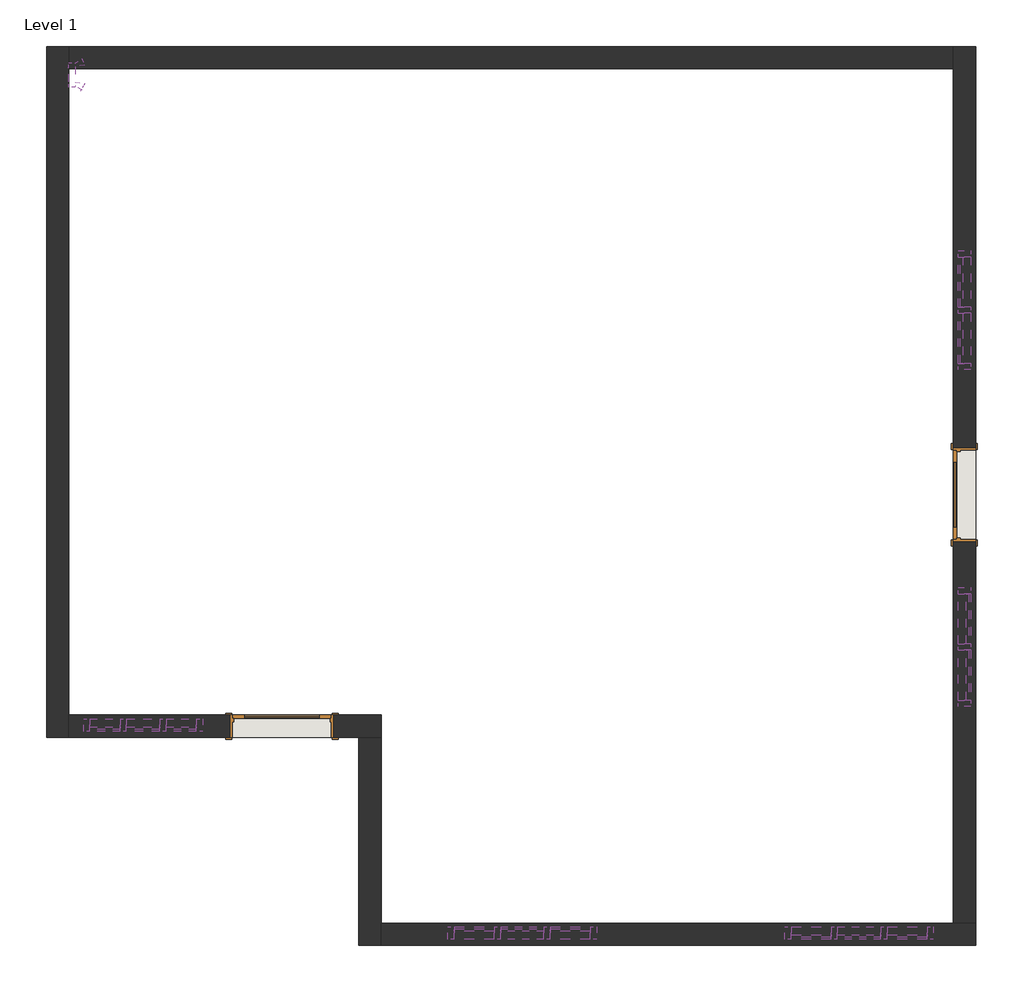
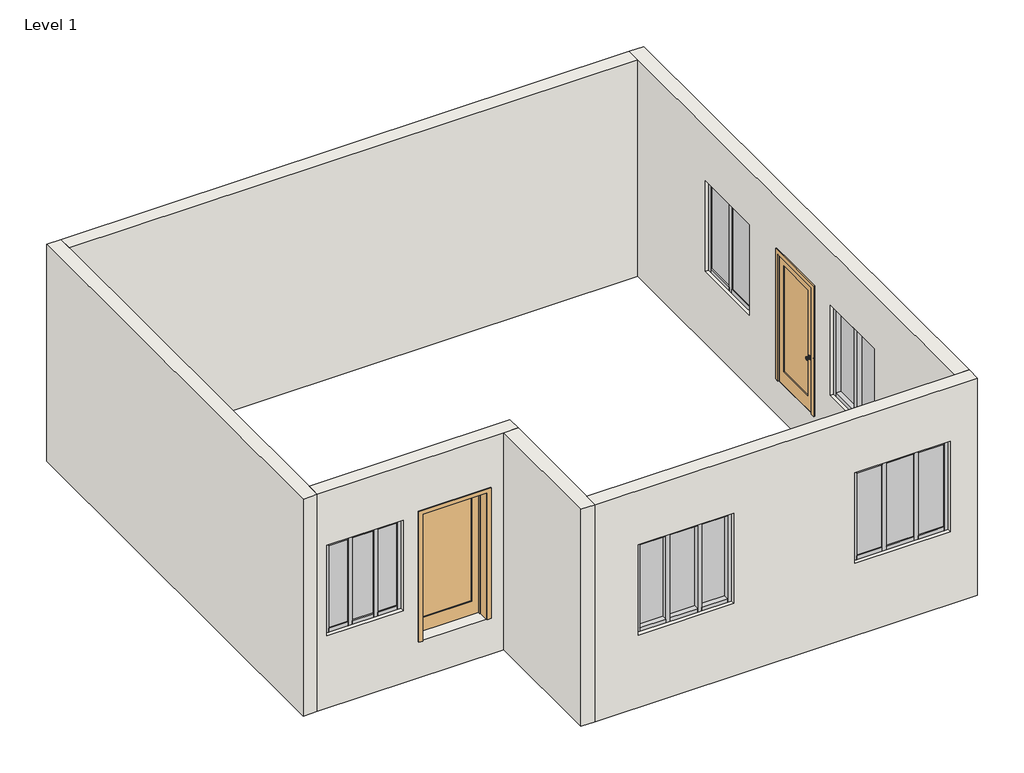
# One storey: 44 members, 13 plates, 6 walls, 2 doors, 1 light fixture.
"""IFC4 building model written with IfcOpenShell, lengths in millimetres."""

from ifc_helpers import new_model, si_unit, frame, origin, place, context, project, spatial, polyline, outline, extrude, faceted_brep, transform, mapped, element, save
from components import door_3b97b8e7, door_3a9a63a9, emergency_wall_light_120v_c8ddf26d, member_5ad95953, member_82905deb, member_ff1b7d8f, member_4491d118, member_dc106669, member_bc7dbe04, member_0b7646a3, system_panel_glazed_3ea5ab3e, system_panel_glazed_321d670a, system_panel_glazed_d22dc6a9, system_panel_glazed_17c4a998, system_panel_glazed_24803b90

model = new_model("IFC4")

# Units and contexts
model_context = context("Model", 3, world=origin())
ifc_project = project(units=[si_unit("LENGTHUNIT", "METRE", prefix="MILLI")], contexts=[model_context])

# Site, building, storey
site = spatial("IfcSite", under=ifc_project)
building = spatial("IfcBuilding", under=site)
storey = spatial("IfcBuildingStorey", under=building, Name="Level 1", Elevation=-609.6)

# Doors
placement = place(None, origin())
door_shape = door_3b97b8e7(model_context)
element("IfcDoor", 1, ObjectType="Door-Interior-Single-1_Panel-Wood : 36\" x 84\" 3", at=placement, inside=storey, context=model_context, shape_type="MappedRepresentation", body=[
    mapped(door_shape, transform((-1873.6852438, 78.3065419, 0.0), x_axis=(0.0, 1.0, 0.0), y_axis=(-1.0, 0.0, 0.0), z_axis=(0.0, 0.0, 1.0))),
])
door_2_shape = door_3a9a63a9(model_context)
element("IfcDoor", 2, ObjectType="Door-Interior-Single-1_Panel-Wood : 40\" x 84\"", at=placement, inside=storey, context=model_context, shape_type="MappedRepresentation", body=[
    mapped(door_2_shape, transform((-8868.2102438, -2293.4184581, 0.0), x_axis=(1.0, 0.0, 0.0), y_axis=(0.0, 1.0, 0.0), z_axis=(0.0, 0.0, 1.0))),
])

# Light fixture
emergency_wall_light_120v_shape = emergency_wall_light_120v_c8ddf26d(model_context)
element("IfcLightFixture", 3, ObjectType="Emergency Wall Light : 120V", at=placement, inside=storey, context=model_context, shape_type="MappedRepresentation", body=[
    mapped(emergency_wall_light_120v_shape, transform((-11195.7738092, 4383.6065419, 301.1463629), x_axis=(0.0, -1.0, 0.0), y_axis=(1.0, 0.0, 0.0), z_axis=(0.0, 0.0, 1.0))),
])

# Members
member_shape = member_5ad95953(model_context)
element("IfcMember", 4, ObjectType="Rectangular Mullion : 2.5\" x 5\" rectangular", at=placement, inside=storey, context=model_context, shape_type="MappedRepresentation", body=[
    mapped(member_shape, transform((-10836.7102438, -2283.8934581, 2133.6), x_axis=(0.0, 0.0, 1.0), y_axis=(0.0, 1.0, 0.0), z_axis=(-1.0, 0.0, 0.0))),
])
element("IfcMember", 5, ObjectType="Rectangular Mullion : 2.5\" x 5\" rectangular", at=placement, inside=storey, context=model_context, shape_type="MappedRepresentation", body=[
    mapped(member_shape, transform((-10055.6602438, -2283.8934581, 2133.6), x_axis=(0.0, 0.0, 1.0), y_axis=(0.0, 1.0, 0.0), z_axis=(-1.0, 0.0, 0.0))),
])
element("IfcMember", 6, ObjectType="Rectangular Mullion : 2.5\" x 5\" rectangular", at=placement, inside=storey, context=model_context, shape_type="MappedRepresentation", body=[
    mapped(member_shape, transform((-9744.5102438, -2283.8934581, 609.6), x_axis=(0.0, 0.0, -1.0), y_axis=(0.0, 1.0, 0.0), z_axis=(1.0, 0.0, 0.0))),
])
element("IfcMember", 7, ObjectType="Rectangular Mullion : 2.5\" x 5\" rectangular", at=placement, inside=storey, context=model_context, shape_type="MappedRepresentation", body=[
    mapped(member_shape, transform((-10525.5602438, -2283.8934581, 609.6), x_axis=(0.0, 0.0, -1.0), y_axis=(0.0, 1.0, 0.0), z_axis=(1.0, 0.0, 0.0))),
])
member_2_shape = member_82905deb(model_context)
element("IfcMember", 8, ObjectType="Rectangular Mullion : 2.5\" x 5\" rectangular", at=placement, inside=storey, context=model_context, shape_type="MappedRepresentation", body=[
    mapped(member_2_shape, transform((-10493.8102438, -2283.8934581, 609.6), x_axis=(-1.0, 0.0, 0.0), y_axis=(0.0, 1.0, 0.0), z_axis=(0.0, 0.0, -1.0))),
])
element("IfcMember", 9, ObjectType="Rectangular Mullion : 2.5\" x 5\" rectangular", at=placement, inside=storey, context=model_context, shape_type="MappedRepresentation", body=[
    mapped(member_2_shape, transform((-10087.4102438, -2283.8934581, 609.6), x_axis=(-1.0, 0.0, 0.0), y_axis=(0.0, 1.0, 0.0), z_axis=(0.0, 0.0, -1.0))),
])
element("IfcMember", 10, ObjectType="Rectangular Mullion : 2.5\" x 5\" rectangular", at=placement, inside=storey, context=model_context, shape_type="MappedRepresentation", body=[
    mapped(member_2_shape, transform((-6658.4102438, -4417.4934581, 609.6), x_axis=(1.0, 0.0, 0.0), y_axis=(0.0, -1.0, 0.0), z_axis=(0.0, 0.0, -1.0))),
])
element("IfcMember", 11, ObjectType="Rectangular Mullion : 2.5\" x 5\" rectangular", at=placement, inside=storey, context=model_context, shape_type="MappedRepresentation", body=[
    mapped(member_2_shape, transform((-6150.4102438, -4417.4934581, 609.6), x_axis=(1.0, 0.0, 0.0), y_axis=(0.0, -1.0, 0.0), z_axis=(0.0, 0.0, -1.0))),
])
element("IfcMember", 12, ObjectType="Rectangular Mullion : 2.5\" x 5\" rectangular", at=placement, inside=storey, context=model_context, shape_type="MappedRepresentation", body=[
    mapped(member_2_shape, transform((-3204.0102438, -4417.4934581, 609.6), x_axis=(-1.0, 0.0, 0.0), y_axis=(0.0, 1.0, 0.0), z_axis=(0.0, 0.0, -1.0))),
])
element("IfcMember", 13, ObjectType="Rectangular Mullion : 2.5\" x 5\" rectangular", at=placement, inside=storey, context=model_context, shape_type="MappedRepresentation", body=[
    mapped(member_2_shape, transform((-2696.0102438, -4417.4934581, 609.6), x_axis=(-1.0, 0.0, 0.0), y_axis=(0.0, 1.0, 0.0), z_axis=(0.0, 0.0, -1.0))),
])
element("IfcMember", 14, ObjectType="Rectangular Mullion : 2.5\" x 5\" rectangular", at=placement, inside=storey, context=model_context, shape_type="MappedRepresentation", body=[
    mapped(member_2_shape, transform((-1870.5102438, -1483.7934581, 609.6), x_axis=(0.0, -1.0, 0.0), y_axis=(-1.0, 0.0, 0.0), z_axis=(0.0, 0.0, -1.0))),
])
element("IfcMember", 15, ObjectType="Rectangular Mullion : 2.5\" x 5\" rectangular", at=placement, inside=storey, context=model_context, shape_type="MappedRepresentation", body=[
    mapped(member_2_shape, transform((-1870.5102438, 1970.6065419, 609.6), x_axis=(0.0, 1.0, 0.0), y_axis=(1.0, 0.0, 0.0), z_axis=(0.0, 0.0, -1.0))),
])
member_3_shape = member_ff1b7d8f(model_context)
element("IfcMember", 16, ObjectType="Rectangular Mullion : 2.5\" x 5\" rectangular", at=placement, inside=storey, context=model_context, shape_type="MappedRepresentation", body=[
    mapped(member_3_shape, transform((-10119.1602438, -2283.8934581, 609.6), x_axis=(0.0, 0.0, -1.0), y_axis=(0.0, 1.0, 0.0), z_axis=(1.0, 0.0, 0.0))),
])
element("IfcMember", 17, ObjectType="Rectangular Mullion : 2.5\" x 5\" rectangular", at=placement, inside=storey, context=model_context, shape_type="MappedRepresentation", body=[
    mapped(member_3_shape, transform((-10462.0602438, -2283.8934581, 2133.6), x_axis=(0.0, 0.0, 1.0), y_axis=(0.0, 1.0, 0.0), z_axis=(-1.0, 0.0, 0.0))),
])
member_4_shape = member_4491d118(model_context)
element("IfcMember", 18, ObjectType="Rectangular Mullion : 2.5\" x 5\" rectangular", at=placement, inside=storey, context=model_context, shape_type="MappedRepresentation", body=[
    mapped(member_4_shape, transform((-9681.0102438, -2283.8934581, 2133.6), x_axis=(1.0, 0.0, 0.0), y_axis=(0.0, 1.0, 0.0), z_axis=(0.0, 0.0, 1.0))),
])
element("IfcMember", 19, ObjectType="Rectangular Mullion : 2.5\" x 5\" rectangular", at=placement, inside=storey, context=model_context, shape_type="MappedRepresentation", body=[
    mapped(member_4_shape, transform((-7166.4102438, -4417.4934581, 2133.6), x_axis=(-1.0, 0.0, 0.0), y_axis=(0.0, -1.0, 0.0), z_axis=(0.0, 0.0, 1.0))),
])
element("IfcMember", 20, ObjectType="Rectangular Mullion : 2.5\" x 5\" rectangular", at=placement, inside=storey, context=model_context, shape_type="MappedRepresentation", body=[
    mapped(member_4_shape, transform((-2188.0102438, -4417.4934581, 2133.6), x_axis=(1.0, 0.0, 0.0), y_axis=(0.0, 1.0, 0.0), z_axis=(0.0, 0.0, 1.0))),
])
element("IfcMember", 21, ObjectType="Rectangular Mullion : 2.5\" x 5\" rectangular", at=placement, inside=storey, context=model_context, shape_type="MappedRepresentation", body=[
    mapped(member_4_shape, transform((-1870.5102438, -874.1934581, 2133.6), x_axis=(0.0, 1.0, 0.0), y_axis=(-1.0, 0.0, 0.0), z_axis=(0.0, 0.0, 1.0))),
])
element("IfcMember", 22, ObjectType="Rectangular Mullion : 2.5\" x 5\" rectangular", at=placement, inside=storey, context=model_context, shape_type="MappedRepresentation", body=[
    mapped(member_4_shape, transform((-1870.5102438, 1361.0065419, 2133.6), x_axis=(0.0, -1.0, 0.0), y_axis=(1.0, 0.0, 0.0), z_axis=(0.0, 0.0, 1.0))),
])
element("IfcMember", 23, ObjectType="Rectangular Mullion : 2.5\" x 5\" rectangular", at=placement, inside=storey, context=model_context, shape_type="MappedRepresentation", body=[
    mapped(member_4_shape, transform((-10900.2102438, -2283.8934581, 609.6), x_axis=(-1.0, 0.0, 0.0), y_axis=(0.0, 1.0, 0.0), z_axis=(0.0, 0.0, -1.0))),
])
element("IfcMember", 24, ObjectType="Rectangular Mullion : 2.5\" x 5\" rectangular", at=placement, inside=storey, context=model_context, shape_type="MappedRepresentation", body=[
    mapped(member_4_shape, transform((-5642.4102438, -4417.4934581, 609.6), x_axis=(1.0, 0.0, 0.0), y_axis=(0.0, -1.0, 0.0), z_axis=(0.0, 0.0, -1.0))),
])
element("IfcMember", 25, ObjectType="Rectangular Mullion : 2.5\" x 5\" rectangular", at=placement, inside=storey, context=model_context, shape_type="MappedRepresentation", body=[
    mapped(member_4_shape, transform((-3712.0102438, -4417.4934581, 609.6), x_axis=(-1.0, 0.0, 0.0), y_axis=(0.0, 1.0, 0.0), z_axis=(0.0, 0.0, -1.0))),
])
element("IfcMember", 26, ObjectType="Rectangular Mullion : 2.5\" x 5\" rectangular", at=placement, inside=storey, context=model_context, shape_type="MappedRepresentation", body=[
    mapped(member_4_shape, transform((-1870.5102438, -2093.3934581, 609.6), x_axis=(0.0, -1.0, 0.0), y_axis=(-1.0, 0.0, 0.0), z_axis=(0.0, 0.0, -1.0))),
])
element("IfcMember", 27, ObjectType="Rectangular Mullion : 2.5\" x 5\" rectangular", at=placement, inside=storey, context=model_context, shape_type="MappedRepresentation", body=[
    mapped(member_4_shape, transform((-1870.5102438, 2580.2065419, 609.6), x_axis=(0.0, 1.0, 0.0), y_axis=(1.0, 0.0, 0.0), z_axis=(0.0, 0.0, -1.0))),
])
member_5_shape = member_dc106669(model_context)
element("IfcMember", 28, ObjectType="Rectangular Mullion : 2.5\" x 5\" rectangular", at=placement, inside=storey, context=model_context, shape_type="MappedRepresentation", body=[
    mapped(member_5_shape, transform((-5705.9102438, -4417.4934581, 2133.6), x_axis=(0.0, 0.0, 1.0), y_axis=(0.0, -1.0, 0.0), z_axis=(1.0, 0.0, 0.0))),
])
element("IfcMember", 29, ObjectType="Rectangular Mullion : 2.5\" x 5\" rectangular", at=placement, inside=storey, context=model_context, shape_type="MappedRepresentation", body=[
    mapped(member_5_shape, transform((-6690.1602438, -4417.4934581, 2133.6), x_axis=(0.0, 0.0, 1.0), y_axis=(0.0, -1.0, 0.0), z_axis=(1.0, 0.0, 0.0))),
])
element("IfcMember", 30, ObjectType="Rectangular Mullion : 2.5\" x 5\" rectangular", at=placement, inside=storey, context=model_context, shape_type="MappedRepresentation", body=[
    mapped(member_5_shape, transform((-3648.5102438, -4417.4934581, 2133.6), x_axis=(0.0, 0.0, 1.0), y_axis=(0.0, 1.0, 0.0), z_axis=(-1.0, 0.0, 0.0))),
])
element("IfcMember", 31, ObjectType="Rectangular Mullion : 2.5\" x 5\" rectangular", at=placement, inside=storey, context=model_context, shape_type="MappedRepresentation", body=[
    mapped(member_5_shape, transform((-2664.2602438, -4417.4934581, 2133.6), x_axis=(0.0, 0.0, 1.0), y_axis=(0.0, 1.0, 0.0), z_axis=(-1.0, 0.0, 0.0))),
])
element("IfcMember", 32, ObjectType="Rectangular Mullion : 2.5\" x 5\" rectangular", at=placement, inside=storey, context=model_context, shape_type="MappedRepresentation", body=[
    mapped(member_5_shape, transform((-7102.9102438, -4417.4934581, 609.6), x_axis=(0.0, 0.0, -1.0), y_axis=(0.0, -1.0, 0.0), z_axis=(-1.0, 0.0, 0.0))),
])
element("IfcMember", 33, ObjectType="Rectangular Mullion : 2.5\" x 5\" rectangular", at=placement, inside=storey, context=model_context, shape_type="MappedRepresentation", body=[
    mapped(member_5_shape, transform((-6118.6602438, -4417.4934581, 609.6), x_axis=(0.0, 0.0, -1.0), y_axis=(0.0, -1.0, 0.0), z_axis=(-1.0, 0.0, 0.0))),
])
element("IfcMember", 34, ObjectType="Rectangular Mullion : 2.5\" x 5\" rectangular", at=placement, inside=storey, context=model_context, shape_type="MappedRepresentation", body=[
    mapped(member_5_shape, transform((-2251.5102438, -4417.4934581, 609.6), x_axis=(0.0, 0.0, -1.0), y_axis=(0.0, 1.0, 0.0), z_axis=(1.0, 0.0, 0.0))),
])
element("IfcMember", 35, ObjectType="Rectangular Mullion : 2.5\" x 5\" rectangular", at=placement, inside=storey, context=model_context, shape_type="MappedRepresentation", body=[
    mapped(member_5_shape, transform((-3235.7602438, -4417.4934581, 609.6), x_axis=(0.0, 0.0, -1.0), y_axis=(0.0, 1.0, 0.0), z_axis=(1.0, 0.0, 0.0))),
])
member_6_shape = member_bc7dbe04(model_context)
element("IfcMember", 36, ObjectType="Rectangular Mullion : 2.5\" x 5\" rectangular", at=placement, inside=storey, context=model_context, shape_type="MappedRepresentation", body=[
    mapped(member_6_shape, transform((-6626.6602438, -4417.4934581, 609.6), x_axis=(0.0, 0.0, -1.0), y_axis=(0.0, -1.0, 0.0), z_axis=(-1.0, 0.0, 0.0))),
])
element("IfcMember", 37, ObjectType="Rectangular Mullion : 2.5\" x 5\" rectangular", at=placement, inside=storey, context=model_context, shape_type="MappedRepresentation", body=[
    mapped(member_6_shape, transform((-2727.7602438, -4417.4934581, 609.6), x_axis=(0.0, 0.0, -1.0), y_axis=(0.0, 1.0, 0.0), z_axis=(1.0, 0.0, 0.0))),
])
element("IfcMember", 38, ObjectType="Rectangular Mullion : 2.5\" x 5\" rectangular", at=placement, inside=storey, context=model_context, shape_type="MappedRepresentation", body=[
    mapped(member_6_shape, transform((-6182.1602438, -4417.4934581, 2133.6), x_axis=(0.0, 0.0, 1.0), y_axis=(0.0, -1.0, 0.0), z_axis=(1.0, 0.0, 0.0))),
])
element("IfcMember", 39, ObjectType="Rectangular Mullion : 2.5\" x 5\" rectangular", at=placement, inside=storey, context=model_context, shape_type="MappedRepresentation", body=[
    mapped(member_6_shape, transform((-3172.2602438, -4417.4934581, 2133.6), x_axis=(0.0, 0.0, 1.0), y_axis=(0.0, 1.0, 0.0), z_axis=(-1.0, 0.0, 0.0))),
])
member_7_shape = member_0b7646a3(model_context)
element("IfcMember", 40, ObjectType="Rectangular Mullion : 2.5\" x 5\" rectangular", at=placement, inside=storey, context=model_context, shape_type="MappedRepresentation", body=[
    mapped(member_7_shape, transform((-1870.5102438, -2029.8934581, 2133.6), x_axis=(0.0, 0.0, 1.0), y_axis=(-1.0, 0.0, 0.0), z_axis=(0.0, -1.0, 0.0))),
])
element("IfcMember", 41, ObjectType="Rectangular Mullion : 2.5\" x 5\" rectangular", at=placement, inside=storey, context=model_context, shape_type="MappedRepresentation", body=[
    mapped(member_7_shape, transform((-1870.5102438, -1452.0434581, 2133.6), x_axis=(0.0, 0.0, 1.0), y_axis=(-1.0, 0.0, 0.0), z_axis=(0.0, -1.0, 0.0))),
])
element("IfcMember", 42, ObjectType="Rectangular Mullion : 2.5\" x 5\" rectangular", at=placement, inside=storey, context=model_context, shape_type="MappedRepresentation", body=[
    mapped(member_7_shape, transform((-1870.5102438, 2516.7065419, 2133.6), x_axis=(0.0, 0.0, 1.0), y_axis=(1.0, 0.0, 0.0), z_axis=(0.0, 1.0, 0.0))),
])
element("IfcMember", 43, ObjectType="Rectangular Mullion : 2.5\" x 5\" rectangular", at=placement, inside=storey, context=model_context, shape_type="MappedRepresentation", body=[
    mapped(member_7_shape, transform((-1870.5102438, 1938.8565419, 2133.6), x_axis=(0.0, 0.0, 1.0), y_axis=(1.0, 0.0, 0.0), z_axis=(0.0, 1.0, 0.0))),
])
element("IfcMember", 44, ObjectType="Rectangular Mullion : 2.5\" x 5\" rectangular", at=placement, inside=storey, context=model_context, shape_type="MappedRepresentation", body=[
    mapped(member_7_shape, transform((-1870.5102438, -937.6934581, 609.6), x_axis=(0.0, 0.0, -1.0), y_axis=(-1.0, 0.0, 0.0), z_axis=(0.0, 1.0, 0.0))),
])
element("IfcMember", 45, ObjectType="Rectangular Mullion : 2.5\" x 5\" rectangular", at=placement, inside=storey, context=model_context, shape_type="MappedRepresentation", body=[
    mapped(member_7_shape, transform((-1870.5102438, -1515.5434581, 609.6), x_axis=(0.0, 0.0, -1.0), y_axis=(-1.0, 0.0, 0.0), z_axis=(0.0, 1.0, 0.0))),
])
element("IfcMember", 46, ObjectType="Rectangular Mullion : 2.5\" x 5\" rectangular", at=placement, inside=storey, context=model_context, shape_type="MappedRepresentation", body=[
    mapped(member_7_shape, transform((-1870.5102438, 1424.5065419, 609.6), x_axis=(0.0, 0.0, -1.0), y_axis=(1.0, 0.0, 0.0), z_axis=(0.0, -1.0, 0.0))),
])
element("IfcMember", 47, ObjectType="Rectangular Mullion : 2.5\" x 5\" rectangular", at=placement, inside=storey, context=model_context, shape_type="MappedRepresentation", body=[
    mapped(member_7_shape, transform((-1870.5102438, 2002.3565419, 609.6), x_axis=(0.0, 0.0, -1.0), y_axis=(1.0, 0.0, 0.0), z_axis=(0.0, -1.0, 0.0))),
])

# Plates
system_panel_glazed_shape = system_panel_glazed_3ea5ab3e(model_context)
element("IfcPlate", 48, ObjectType="System Panel : Glazed", at=placement, inside=storey, context=model_context, shape_type="MappedRepresentation", body=[
    mapped(system_panel_glazed_shape, transform((-9900.0852438, -2283.8934581, 673.1), x_axis=(-1.0, 0.0, 0.0), y_axis=(0.0, -1.0, 0.0), z_axis=(0.0, 0.0, 1.0))),
])
element("IfcPlate", 49, ObjectType="System Panel : Glazed", at=placement, inside=storey, context=model_context, shape_type="MappedRepresentation", body=[
    mapped(system_panel_glazed_shape, transform((-10681.1352438, -2283.8934581, 673.1), x_axis=(-1.0, 0.0, 0.0), y_axis=(0.0, -1.0, 0.0), z_axis=(0.0, 0.0, 1.0))),
])
system_panel_glazed_2_shape = system_panel_glazed_321d670a(model_context)
element("IfcPlate", 50, ObjectType="System Panel : Glazed", at=placement, inside=storey, context=model_context, shape_type="MappedRepresentation", body=[
    mapped(system_panel_glazed_2_shape, transform((-10290.6102438, -2283.8934581, 673.1), x_axis=(-1.0, 0.0, 0.0), y_axis=(0.0, -1.0, 0.0), z_axis=(0.0, 0.0, 1.0))),
])
system_panel_glazed_3_shape = system_panel_glazed_d22dc6a9(model_context)
element("IfcPlate", 51, ObjectType="System Panel : Glazed", at=placement, inside=storey, context=model_context, shape_type="MappedRepresentation", body=[
    mapped(system_panel_glazed_3_shape, transform((-6896.5352438, -4417.4934581, 673.1), x_axis=(1.0, 0.0, 0.0), y_axis=(0.0, 1.0, 0.0), z_axis=(0.0, 0.0, 1.0))),
])
element("IfcPlate", 52, ObjectType="System Panel : Glazed", at=placement, inside=storey, context=model_context, shape_type="MappedRepresentation", body=[
    mapped(system_panel_glazed_3_shape, transform((-2457.8852438, -4417.4934581, 673.1), x_axis=(-1.0, 0.0, 0.0), y_axis=(0.0, -1.0, 0.0), z_axis=(0.0, 0.0, 1.0))),
])
element("IfcPlate", 53, ObjectType="System Panel : Glazed", at=placement, inside=storey, context=model_context, shape_type="MappedRepresentation", body=[
    mapped(system_panel_glazed_3_shape, transform((-5912.2852438, -4417.4934581, 673.1), x_axis=(1.0, 0.0, 0.0), y_axis=(0.0, 1.0, 0.0), z_axis=(0.0, 0.0, 1.0))),
])
element("IfcPlate", 54, ObjectType="System Panel : Glazed", at=placement, inside=storey, context=model_context, shape_type="MappedRepresentation", body=[
    mapped(system_panel_glazed_3_shape, transform((-3442.1352438, -4417.4934581, 673.1), x_axis=(-1.0, 0.0, 0.0), y_axis=(0.0, -1.0, 0.0), z_axis=(0.0, 0.0, 1.0))),
])
system_panel_glazed_4_shape = system_panel_glazed_17c4a998(model_context)
element("IfcPlate", 55, ObjectType="System Panel : Glazed", at=placement, inside=storey, context=model_context, shape_type="MappedRepresentation", body=[
    mapped(system_panel_glazed_4_shape, transform((-6404.4102438, -4417.4934581, 673.1), x_axis=(1.0, 0.0, 0.0), y_axis=(0.0, 1.0, 0.0), z_axis=(0.0, 0.0, 1.0))),
])
element("IfcPlate", 56, ObjectType="System Panel : Glazed", at=placement, inside=storey, context=model_context, shape_type="MappedRepresentation", body=[
    mapped(system_panel_glazed_4_shape, transform((-2950.0102438, -4417.4934581, 673.1), x_axis=(-1.0, 0.0, 0.0), y_axis=(0.0, -1.0, 0.0), z_axis=(0.0, 0.0, 1.0))),
])
system_panel_glazed_5_shape = system_panel_glazed_24803b90(model_context)
element("IfcPlate", 57, ObjectType="System Panel : Glazed", at=placement, inside=storey, context=model_context, shape_type="MappedRepresentation", body=[
    mapped(system_panel_glazed_5_shape, transform((-1870.5102438, -1194.8684581, 673.1), x_axis=(0.0, -1.0, 0.0), y_axis=(1.0, 0.0, 0.0), z_axis=(0.0, 0.0, 1.0))),
])
element("IfcPlate", 58, ObjectType="System Panel : Glazed", at=placement, inside=storey, context=model_context, shape_type="MappedRepresentation", body=[
    mapped(system_panel_glazed_5_shape, transform((-1870.5102438, 1681.6815419, 673.1), x_axis=(0.0, 1.0, 0.0), y_axis=(-1.0, 0.0, 0.0), z_axis=(0.0, 0.0, 1.0))),
])
element("IfcPlate", 59, ObjectType="System Panel : Glazed", at=placement, inside=storey, context=model_context, shape_type="MappedRepresentation", body=[
    mapped(system_panel_glazed_5_shape, transform((-1870.5102438, -1772.7184581, 673.1), x_axis=(0.0, -1.0, 0.0), y_axis=(1.0, 0.0, 0.0), z_axis=(0.0, 0.0, 1.0))),
])
element("IfcPlate", 60, ObjectType="System Panel : Glazed", at=placement, inside=storey, context=model_context, shape_type="MappedRepresentation", body=[
    mapped(system_panel_glazed_5_shape, transform((-1870.5102438, 2259.5315419, 673.1), x_axis=(0.0, 1.0, 0.0), y_axis=(-1.0, 0.0, 0.0), z_axis=(0.0, 0.0, 1.0))),
])

# Walls
element("IfcWall", 61, ObjectType="9\" wall", at=placement, inside=storey, context=model_context, shape_type="Brep", body=[
    faceted_brep([(-11281.2102438, 4675.7065419, -609.6), (-11281.2102438, -2410.8934581, -609.6), (-11281.2102438, -2410.8934581, 3048.0), (-11281.2102438, 4675.7065419, 3048.0), (-11052.6102438, 4675.7065419, -609.6), (-11052.6102438, 4675.7065419, 3048.0), (-11052.6102438, 4447.1065419, 3048.0), (-11052.6102438, -2182.2934581, 3048.0), (-11052.6102438, -2410.8934581, 3048.0), (-11052.6102438, -2410.8934581, -609.6), (-11052.6102438, -2182.2934581, -609.6), (-11052.6102438, 4447.1065419, -609.6)], [[[0, 1, 2, 3]], [[4, 5, 6, 7, 8, 9, 10, 11]], [[1, 0, 4, 11, 10, 9]], [[3, 2, 8, 7, 6, 5]], [[2, 1, 9, 8]], [[0, 3, 5, 4]]]),
])
element("IfcWall", 62, ObjectType="9\" wall", at=placement, inside=storey, context=model_context, shape_type="Brep", body=[
    faceted_brep([(-11052.6102438, -2410.8934581, -609.6), (-8080.8102438, -2410.8934581, -609.6), (-7852.2102438, -2410.8934581, -609.6), (-7852.2102438, -2410.8934581, 3048.0), (-8080.8102438, -2410.8934581, 3048.0), (-11052.6102438, -2410.8934581, 3048.0), (-8334.8102438, -2410.8934581, 2159.0), (-8334.8102438, -2410.8934581, 0.0), (-9401.6102438, -2410.8934581, 0.0), (-9401.6102438, -2410.8934581, 2159.0), (-9681.0102438, -2410.8934581, 2133.6), (-9681.0102438, -2410.8934581, 609.6), (-10900.2102438, -2410.8934581, 609.6), (-10900.2102438, -2410.8934581, 2133.6), (-7852.2102438, -2182.2934581, -609.6), (-11052.6102438, -2182.2934581, -609.6), (-11052.6102438, -2182.2934581, 3048.0), (-7852.2102438, -2182.2934581, 3048.0), (-8334.8102438, -2182.2934581, 0.0), (-8334.8102438, -2182.2934581, 2159.0), (-9401.6102438, -2182.2934581, 2159.0), (-9401.6102438, -2182.2934581, 0.0), (-9681.0102438, -2182.2934581, 609.6), (-9681.0102438, -2182.2934581, 2133.6), (-10900.2102438, -2182.2934581, 2133.6), (-10900.2102438, -2182.2934581, 609.6)], [[[0, 1, 2, 3, 4, 5], [6, 7, 8, 9], [10, 11, 12, 13]], [[14, 15, 16, 17], [18, 19, 20, 21], [22, 23, 24, 25]], [[2, 1, 0, 15, 14]], [[5, 4, 3, 17, 16]], [[0, 5, 16, 15]], [[3, 2, 14, 17]], [[18, 7, 6, 19]], [[19, 6, 9, 20]], [[20, 9, 8, 21]], [[7, 18, 21, 8]], [[10, 23, 22, 11]], [[23, 10, 13, 24]], [[24, 13, 12, 25]], [[11, 22, 25, 12]]]),
])
element("IfcWall", 63, ObjectType="9\" wall", at=placement, inside=storey, context=model_context, shape_type="Brep", body=[
    faceted_brep([(-8080.8102438, -2410.8934581, -609.6), (-8080.8102438, -4544.4934581, -609.6), (-8080.8102438, -4544.4934581, 3048.0), (-8080.8102438, -2410.8934581, 3048.0), (-7852.2102438, -2410.8934581, -609.6), (-7852.2102438, -2410.8934581, 3048.0), (-7852.2102438, -4315.8934581, 3048.0), (-7852.2102438, -4544.4934581, 3048.0), (-7852.2102438, -4544.4934581, -609.6), (-7852.2102438, -4315.8934581, -609.6)], [[[0, 1, 2, 3]], [[4, 5, 6, 7, 8, 9]], [[1, 0, 4, 9, 8]], [[3, 2, 7, 6, 5]], [[0, 3, 5, 4]], [[2, 1, 8, 7]]]),
])
element("IfcWall", 64, ObjectType="9\" wall", at=placement, inside=storey, context=model_context, shape_type="Brep", body=[
    faceted_brep([(-7852.2102438, -4544.4934581, -609.6), (-1756.2102438, -4544.4934581, -609.6), (-1756.2102438, -4544.4934581, 3048.0), (-7852.2102438, -4544.4934581, 3048.0), (-7166.4102438, -4544.4934581, 609.6), (-7166.4102438, -4544.4934581, 2133.6), (-5642.4102438, -4544.4934581, 2133.6), (-5642.4102438, -4544.4934581, 609.6), (-2188.0102438, -4544.4934581, 2133.6), (-2188.0102438, -4544.4934581, 609.6), (-3712.0102438, -4544.4934581, 609.6), (-3712.0102438, -4544.4934581, 2133.6), (-1756.2102438, -4315.8934581, -609.6), (-1984.8102438, -4315.8934581, -609.6), (-7852.2102438, -4315.8934581, -609.6), (-7852.2102438, -4315.8934581, 3048.0), (-1984.8102438, -4315.8934581, 3048.0), (-1756.2102438, -4315.8934581, 3048.0), (-7166.4102438, -4315.8934581, 2133.6), (-7166.4102438, -4315.8934581, 609.6), (-5642.4102438, -4315.8934581, 609.6), (-5642.4102438, -4315.8934581, 2133.6), (-2188.0102438, -4315.8934581, 609.6), (-2188.0102438, -4315.8934581, 2133.6), (-3712.0102438, -4315.8934581, 2133.6), (-3712.0102438, -4315.8934581, 609.6)], [[[0, 1, 2, 3], [4, 5, 6, 7], [8, 9, 10, 11]], [[12, 13, 14, 15, 16, 17], [18, 19, 20, 21], [22, 23, 24, 25]], [[1, 0, 14, 13, 12]], [[3, 2, 17, 16, 15]], [[2, 1, 12, 17]], [[18, 5, 4, 19]], [[5, 18, 21, 6]], [[6, 21, 20, 7]], [[19, 4, 7, 20]], [[22, 9, 8, 23]], [[23, 8, 11, 24]], [[24, 11, 10, 25]], [[9, 22, 25, 10]], [[0, 3, 15, 14]]]),
])
element("IfcWall", 65, ObjectType="9\" wall", at=placement, inside=storey, context=model_context, shape_type="Brep", body=[
    faceted_brep([(-1756.2102438, -4315.8934581, -609.6), (-1756.2102438, 4675.7065419, -609.6), (-1756.2102438, 4675.7065419, 3048.0), (-1756.2102438, -4315.8934581, 3048.0), (-1756.2102438, 560.9065419, 2159.0), (-1756.2102438, 560.9065419, 0.0), (-1756.2102438, -404.2934581, 0.0), (-1756.2102438, -404.2934581, 2159.0), (-1756.2102438, 1361.0065419, 609.6), (-1756.2102438, 1361.0065419, 2133.6), (-1756.2102438, 2580.2065419, 2133.6), (-1756.2102438, 2580.2065419, 609.6), (-1756.2102438, -874.1934581, 2133.6), (-1756.2102438, -874.1934581, 609.6), (-1756.2102438, -2093.3934581, 609.6), (-1756.2102438, -2093.3934581, 2133.6), (-1984.8102438, 4675.7065419, -609.6), (-1984.8102438, 4447.1065419, -609.6), (-1984.8102438, -4315.8934581, -609.6), (-1984.8102438, -4315.8934581, 3048.0), (-1984.8102438, 4447.1065419, 3048.0), (-1984.8102438, 4675.7065419, 3048.0), (-1984.8102438, 560.9065419, 0.0), (-1984.8102438, 560.9065419, 2159.0), (-1984.8102438, -404.2934581, 2159.0), (-1984.8102438, -404.2934581, 0.0), (-1984.8102438, 1361.0065419, 2133.6), (-1984.8102438, 1361.0065419, 609.6), (-1984.8102438, 2580.2065419, 609.6), (-1984.8102438, 2580.2065419, 2133.6), (-1984.8102438, -874.1934581, 609.6), (-1984.8102438, -874.1934581, 2133.6), (-1984.8102438, -2093.3934581, 2133.6), (-1984.8102438, -2093.3934581, 609.6)], [[[0, 1, 2, 3], [4, 5, 6, 7], [8, 9, 10, 11], [12, 13, 14, 15]], [[16, 17, 18, 19, 20, 21], [22, 23, 24, 25], [26, 27, 28, 29], [30, 31, 32, 33]], [[1, 0, 18, 17, 16]], [[3, 2, 21, 20, 19]], [[0, 3, 19, 18]], [[2, 1, 16, 21]], [[22, 5, 4, 23]], [[23, 4, 7, 24]], [[24, 7, 6, 25]], [[5, 22, 25, 6]], [[26, 9, 8, 27]], [[9, 26, 29, 10]], [[10, 29, 28, 11]], [[27, 8, 11, 28]], [[12, 31, 30, 13]], [[31, 12, 15, 32]], [[32, 15, 14, 33]], [[13, 30, 33, 14]]]),
])
element("IfcWall", 66, ObjectType="9\" wall", at=placement, inside=storey, context=model_context, shape_type="SweptSolid", body=[
    extrude(outline(polyline([(-11052.6102438, 4675.7065419), (-1984.8102438, 4675.7065419), (-1984.8102438, 4447.1065419), (-11052.6102438, 4447.1065419), (-11052.6102438, 4675.7065419)])), frame((0.0, 0.0, -609.6), z_axis=(0.0, 0.0, 1.0), x_axis=(1.0, 0.0, 0.0)), (0.0, 0.0, 1.0), 3657.6),
])

save(model, "model.ifc")

# Revit data of these elements
# Type "Door-Interior-Single-1_Panel-Wood : 36\" x 84\" 3"
#   Type Mark = "10"
#   Assembly Code = "C1020300"
#   Analytic Construction = "Wooden"
#   Top Rail = 0' - 4 11/16"
#   Thickness = 0' - 1 3/8"
#   Thermal Resistance (R) = 2.5876 (h·ft²·°F)/BTU
#   Swing Angle [instance default] = 90.00°
#   Stiles = 0' - 4 3/4"
#   Rough Width = 3' - 2"
#   Rough Height = 7' - 1"
#   Height = 7' - 0"
#   Width = 3' - 0"
#   Heat Transfer Coefficient (U) = 0.3865 BTU/(h·ft²·°F)
#   Bottom Rail = 0' - 9 1/8"
#   Trim Material = door
#   Panel Material = door
#   Frame Material = door
#   Door Handle Material = Aluminum
#   Visual Light Transmittance = 0
#   Solar Heat Gain Coefficient = 0
#   Wall Closure = (empty or 0)
#   Function = (empty or 0)
# Type "Door-Interior-Single-1_Panel-Wood : 40\" x 84\""
#   Type Mark = "9"
#   Assembly Code = "C1020300"
#   Analytic Construction = "Wooden"
#   Top Rail = 0' - 4 11/16"
#   Thickness = 0' - 1 3/8"
#   Thermal Resistance (R) = 2.5876 (h·ft²·°F)/BTU
#   Swing Angle [instance default] = 90.00°
#   Stiles = 0' - 4 3/4"
#   Rough Width = 3' - 6"
#   Rough Height = 7' - 1"
#   Height = 7' - 0"
#   Width = 3' - 4"
#   Heat Transfer Coefficient (U) = 0.3865 BTU/(h·ft²·°F)
#   Bottom Rail = 0' - 9 1/8"
#   Trim Material = Cherry
#   Panel Material = door
#   Frame Material = Cherry
#   Door Handle Material = Aluminum
#   Visual Light Transmittance = 0
#   Solar Heat Gain Coefficient = 0
#   Wall Closure = (empty or 0)
#   Function = (empty or 0)
# Type "Emergency Wall Light : 120V"
#   Lamp = "A-19"
#   Assembly Code = "D5090200"
#   Wattage Comments = "100"
#   Ballast Voltage = 120 V
#   Mounting Height = 7' - 0"
#   Apparent Load = 100 VA
#   Ballast Number of Poles = 1
#   Diffuser = Glass, White, High Luminance
#   Light Casing = Steel, Paint Finish, Ivory, Glossy
#   Default Elevation = 0
# Type "Rectangular Mullion : 2.5\" x 5\" rectangular"
#   built-in parameter 1007304 = 0.416667 (stored number, unit not read)
#   built-in parameter 1007301 = 0.104167 (stored number, unit not read)
#   built-in parameter 1007300 = 0.104167 (stored number, unit not read)
# Type "System Panel : Glazed"
#   Construction Type Id = "GSP4R"
#   Analytic Construction = "1/8 in Pilkington single glazing"
#   Visual Light Transmittance = 0.9
#   Solar Heat Gain Coefficient = 0.86
#   Heat Transfer Coefficient (U) = 1.18115 BTU/(h·ft²·°F)
#   Define Thermal Properties by = 1
# Type "9\" wall"
#   Assembly Code = "B2010"
#   Layers, outside or top first: 0' - 9" "Gypsum Wall Board" (function 1)
# Element 1 (IfcDoor, "Door-Interior-Single-1_Panel-Wood : 36\" x 84\" 3")
#   Swing Angle = 90.00°
#   Phase Created = New Construction
#   Materials on its faces: "door", "Aluminum"
# Element 2 (IfcDoor, "Door-Interior-Single-1_Panel-Wood : 40\" x 84\"")
#   Swing Angle = 90.00°
#   Phase Created = New Construction
#   Materials on its faces: "Cherry", "Aluminum", "door"
# Element 3 (IfcLightFixture, "Emergency Wall Light : 120V")
#   Mark = "3"
#   Phase Created = New Construction
#   Materials on its faces: "Steel, Paint Finish, Ivory, Glossy", "Glass, White, High Luminance"
# Elements 4, 5, 6, 7, 8, 9, 10, 11, 12, 13, 14, 15, 16, 17, 18, 19, 20, 21, 22, 23, 24, 25, 26, 27, 28, 29, 30, 31, 32, 33, 34, 35, 36, 37, 38, 39, 40, 41, 42, 43, 44, 45, 46, 47 (IfcMember, "Rectangular Mullion : 2.5\" x 5\" rectangular")
#   Phase Created = New Construction
# Elements 48, 49, 50, 51, 52, 53, 54, 55, 56, 57, 58, 59, 60 (IfcPlate, "System Panel : Glazed")
#   Phase Created = New Construction
#   Materials on its faces: "Glass"
# Elements 61, 62, 63, 64, 65, 66 (IfcWall, "9\" wall")
#   Top Offset = 0' - 0"
#   Base Offset = 0' - 0"
#   wall height = 12' - 0"
#   Phase Created = New Construction
#   Base Constraint = Level 1
#   Top Constraint = Level 2
#   Materials on its faces: "Gypsum Wall Board"
# Materials
#   "door": class "Generic", colour RGB 120 120 120, transparency 0, Cost = 0
#   "Aluminum": class "Metal", colour RGB 247 247 247, transparency 0, Description = "Aluminum 6061", Cost = 0
#   "Cherry": class "Wood", colour RGB 226 177 128, transparency 0, Description = "Prunus Serotina", Cost = 0
#   "Glass, White, High Luminance": class "Glass", colour RGB 249 250 249, transparency 0.8, Description = "physical material", Cost = 0
#   "Steel, Paint Finish, Ivory, Glossy": class "Metal", colour RGB 247 247 239, transparency 0, Description = "Steel, paint finish, ivory, glossy", Cost = 0
#   "Gypsum Wall Board": class "Generic", colour RGB 127 127 127, transparency 0, Description = "Gypsum Wall Board", Cost = 0
#   "Glass": class "Glass", colour RGB 0 128 192, transparency 0.75, Description = "Soda Lime Glass", Cost = 0
